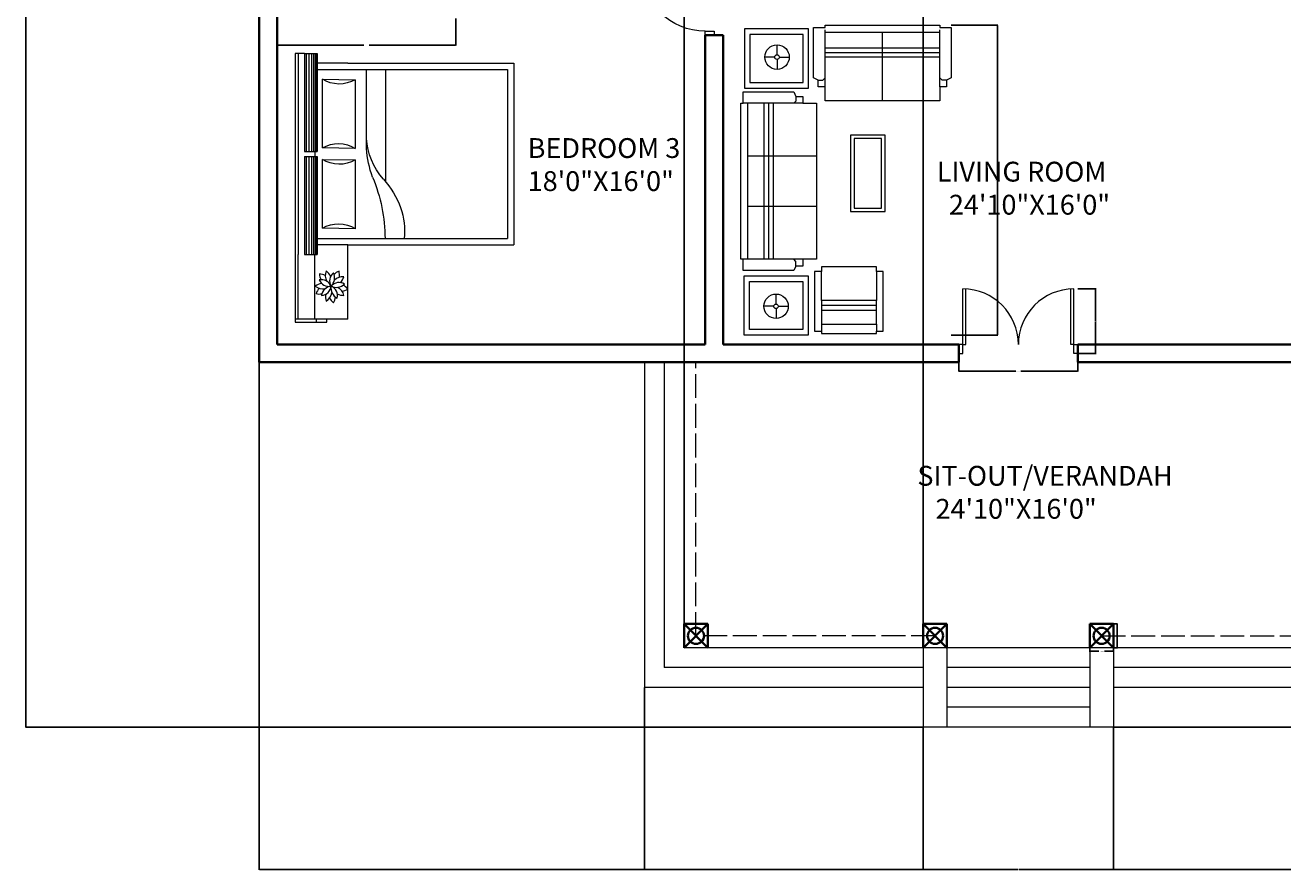
# Model space of a CAD drawing. Units: inches. Extents: x 4602 to 5612, y 5125 to 6591.
# Tile 1 of 6: x 4602 to 5237, y 5125 to 5551. Entities that reach past the tile are written whole.
import ezdxf

# ---------------------------------------------------------------- set-up
doc = ezdxf.new("R2010")
doc.units = ezdxf.units.IN
doc.linetypes.add('ACAD_ISO02W100', pattern=[15, 12, -3])
for name, color, linetype, lineweight in [('A-ANNO-DIMS', 2, 'Continuous', 18), ('A-AREA-IDEN', 7, 'Continuous', 18), ('A-COLS', 7, 'Continuous', 35), ('A-DOOR', 4, 'Continuous', 18), ('A-FLOR-EDGE', 7, 'Continuous', 18), ('A-FLOR-OVHD', 8, 'ACAD_ISO02W100', 13), ('A-FLOR-STRS', 7, 'Continuous', 18), ('A-FURN', 8, 'Continuous', 13), ('A-WALL', 7, 'Continuous', 35)]:
    doc.layers.add(name, color=color, linetype=linetype, lineweight=lineweight)
doc.styles.get("Standard").update_dxf_attribs({"font": 'arial.ttf'})
doc.dimstyles.get("Standard").update_dxf_attribs({"dimtxt": 0.18, "dimasz": 0.18, "dimexe": 0.18, "dimexo": 0.0625, "dimgap": 0.09, "dimtad": 0, "dimtih": 1, "dimtoh": 1, "dimdec": 4, "dimzin": 0, "dimdsep": 46, "dimtxsty": 'Standard', "dimcen": 0.09, "dimadec": 0, "dimazin": 0, "dimtfac": 1, "dimtdec": 4, "dimtofl": 0, "dimtmove": 0, "dimatfit": 3, "dimfxl": 1, "dimtolj": 1, "dimtzin": 0, "dimarcsym": 0})

# ---------------------------------------------------------------- blocks, each defined once
blk = doc.blocks.new('A$C1C981678')
for p, q in [((0, 1425), (0, 2066)), ((0, 2066), (591, 2066)), ((55, 1480), (55, 2011)), ((55, 2011), (536, 2011)), ((536, 2011), (536, 1480)), ((591, 2066), (591, 1425)), ((643, 1571), (643, 2074)), ((643, 2074), (757, 2074)), ((757, 2097), (2312, 2097)), ((757, 2074), (757, 2097)), ((757, 1571), (757, 2074)), ((757, 2028), (2312, 2028)), ((1283, 1342), (1283, 2028)), ((1786, 1342), (1786, 2028)), ((2312, 2097), (2312, 2074)), ((2312, 2074), (2426, 2074)), ((2312, 1571), (2312, 2074)), ((2426, 2074), (2426, 1571)), ((2463, 2062), (2463, 1422)), ((3055, 2062), (2463, 2062)), ((3055, 1422), (3055, 2062)), ((2519, 2007), (2519, 1477)), ((3000, 2007), (2519, 2007)), ((3000, 1477), (3000, 2007)), ((287, 1770), (287, 1869)), ((2312, 1868), (757, 1868)), ((2312, 1822), (757, 1822)), ((2312, 1777), (757, 1777)), ((2773, 1759), (2773, 1859)), ((264, 1747), (165, 1747)), ((287, 1724), (287, 1625)), ((310, 1747), (409, 1747)), ((2750, 1737), (2651, 1737)), ((2773, 1714), (2773, 1615)), ((2796, 1737), (2895, 1737)), ((689, 1548), (643, 1571)), ((689, 1479), (689, 1548)), ((689, 1548), (734, 1548)), ((734, 1548), (757, 1571)), ((757, 1479), (757, 1571)), ((2335, 1548), (2312, 1571)), ((2312, 1479), (2312, 1571)), ((2380, 1548), (2335, 1548)), ((2426, 1571), (2380, 1548)), ((2380, 1548), (2380, 1479)), ((591, 1425), (0, 1425)), ((536, 1480), (55, 1480)), ((757, 1479), (689, 1479)), ((757, 1342), (757, 1479)), ((2380, 1479), (2312, 1479)), ((2312, 1479), (2312, 1342)), ((2463, 1422), (3055, 1422)), ((2519, 1477), (3000, 1477)), ((17, 1295), (17, 746)), ((40, 1295), (17, 1295)), ((634, 1364), (40, 1364)), ((40, 1364), (40, 1295)), ((108, 1295), (40, 1295)), ((345, 1295), (108, 1295)), ((108, 1295), (108, 746)), ((245, 746), (245, 1295)), ((295, 746), (295, 1295)), ((345, 746), (345, 1295)), ((345, 1295), (634, 1295)), ((634, 1295), (634, 1364)), ((680, 1295), (634, 1295)), ((680, 746), (680, 1295)), ((2312, 1342), (757, 1342)), ((2337, 114), (2337, 1257)), ((2337, 1257), (2475, 1257)), ((2475, 1326), (2543, 1326)), ((2475, 1257), (2475, 1326)), ((2475, 1257), (2566, 1257)), ((2543, 1326), (2566, 1372)), ((2543, 1326), (2543, 1280)), ((2543, 1280), (2566, 1257)), ((2566, 1372), (3069, 1372)), ((2566, 1257), (3046, 1257)), ((2772, 114), (2772, 1257)), ((2817, 114), (2817, 1257)), ((2863, 114), (2863, 1257)), ((3023, 1257), (3023, 114)), ((3069, 1372), (3069, 1257)), ((3069, 1257), (3092, 1257)), ((3092, 1257), (3092, 114)), ((1995, 1003), (1232, 1003)), ((1232, 1003), (1232, 659)), ((1960, 969), (1266, 969)), ((1266, 969), (1266, 694)), ((1960, 694), (1960, 969)), ((1995, 659), (1995, 1003)), ((17, 746), (40, 746)), ((40, 746), (40, 678)), ((108, 746), (40, 746)), ((40, 678), (634, 678)), ((108, 746), (345, 746)), ((634, 746), (345, 746)), ((634, 746), (680, 746)), ((634, 678), (634, 746)), ((1232, 659), (1995, 659)), ((1266, 694), (1960, 694)), ((2337, 686), (3023, 686)), ((2475, 114), (2337, 114)), ((2475, 46), (2475, 114)), ((2475, 114), (2566, 114)), ((2543, 46), (2475, 46)), ((2543, 91), (2566, 114)), ((2543, 46), (2543, 91)), ((2566, 0), (2543, 46)), ((2566, 114), (3046, 114)), ((3069, 0), (2566, 0)), ((3092, 114), (3069, 114)), ((3069, 114), (3069, 0))]:
    blk.add_line(p, q)
for radius in [122, 22.9]:
    blk.add_circle((2773, 1737), radius)
for major_axis in [(-86.2, 86.2), (16.2, 16.2)]:
    blk.add_ellipse((287, 1747), major_axis=major_axis, ratio=1)
blk = doc.blocks.new('DOOR-PAIR-60IN')
for p, q in [((2, 4.5), (2, 32.5)), ((3.5, 4.5), (3.5, 32.46)), ((56.5, 4.5), (56.5, 32.46)), ((58, 4.5), (58, 32.5)), ((2, 4.5), (0, 4.5)), ((2, 0), (2, 4.5)), ((2, 4.5), (3.5, 4.5)), ((58, 4.5), (56.5, 4.5)), ((58, 0), (58, 4.5)), ((58, 4.5), (60, 4.5)), ((0, 0), (2, 0)), ((60, 0), (58, 0))]:
    blk.add_line(p, q)
for centre, start, end in [((2, 4.5), 0, 90), ((58, 4.5), 90, 180)]:
    blk.add_arc(centre, 28, start, end)
blk = doc.blocks.new('DOOR-36IN-DEEP-JAMB')
for p, q in [((2, 4.5), (2, 36.5)), ((3.5, 4.5), (3.5, 36.46)), ((0, 4.5), (2, 4.5)), ((2, 4.5), (2, 0)), ((2, 4.5), (3.5, 4.5)), ((36, 4.5), (34, 4.5)), ((34, 4.5), (34, 0)), ((2, 0), (0, 0)), ((34, 0), (36, 0))]:
    blk.add_line(p, q)
blk.add_arc((2, 4.5), 32, 0, 90)
blk = doc.blocks.new('POST-POOMUKHAM')
for p, q in [((12, 12), (0, 12)), ((0, 12), (0, 0)), ((12, 0), (0, 12)), ((0, 0), (12, 12)), ((12, 0), (12, 12))]:
    blk.add_line(p, q)
blk.add_circle((6, 6), 4.06)
blk = doc.blocks.new('BED-DOUBLE')
for p, q in [((0, 108.76), (49.36, 108.76)), ((49.36, 108.76), (52.03, 108.76)), ((52.03, 110.36), (101.4, 110.36)), ((52.03, 108.76), (101.4, 108.76)), ((0, 105.55), (49.36, 105.55)), ((0, 105.55), (0, 99.15)), ((0, 104.75), (49.36, 104.75)), ((0, 103.35), (49.36, 103.35)), ((0, 102.06), (49.36, 102.06)), ((49.36, 105.55), (49.36, 99.15)), ((52.03, 105.55), (52.03, 99.15)), ((52.03, 105.55), (101.4, 105.55)), ((52.03, 104.75), (101.4, 104.75)), ((52.03, 103.35), (101.4, 103.35)), ((52.03, 102.06), (101.4, 102.06)), ((101.4, 105.55), (101.4, 99.15)), ((0, 101), (49.36, 101)), ((0, 100.18), (49.36, 100.18)), ((0, 99.59), (49.36, 99.59)), ((0, 99.15), (49.36, 99.15)), ((4.8, 83.67), (4.8, 99.15)), ((8.01, 99.15), (8.01, 3.2)), ((47.64, 96.58), (12.95, 96.58)), ((12.95, 96.58), (13.21, 79.95)), ((47.9, 79.95), (47.64, 96.58)), ((49.36, 100.32), (52.03, 100.32)), ((52.03, 101), (101.4, 101)), ((52.03, 100.18), (101.4, 100.18)), ((52.03, 99.59), (101.4, 99.59)), ((52.03, 99.15), (101.4, 99.15)), ((88.11, 96.58), (53.42, 96.58)), ((53.42, 96.58), (53.67, 79.95)), ((88.36, 79.95), (88.11, 96.58)), ((93.39, 99.15), (93.39, 3.2)), ((96.59, 83.67), (96.59, 99.15)), ((4.8, 83.67), (4.8, 0)), ((96.59, 83.67), (96.59, 0)), ((13.21, 79.95), (47.9, 79.95)), ((53.67, 79.95), (88.36, 79.95)), ((48.03, 74.3), (8.01, 74.3)), ((64.45, 64.53), (8.01, 64.53)), ((4.8, 0), (96.59, 0)), ((8.01, 3.2), (93.39, 3.2))]:
    blk.add_line(p, q)
for centre, start, end in [((-0.76, 88.06), 329.87223, 31.87128), ((61.61, 88.48), 149.87223, 211.87128), ((39.71, 88.06), 329.87223, 31.87128), ((102.07, 88.48), 149.87223, 211.87128)]:
    blk.add_arc(centre, 16.15, start, end)
for centre, major_axis, ratio, start_param, end_param in [((41.23, 29.43), (0, -44.91), 0.84, 2.512571, 3.097265), ((44.48, 1.25), (0, -73.18), 0.84, 2.845884, 3.083884), ((93.61, 177.65), (0, -112.7), 0.84, -0.336035, -0.002349), ((86.52, 99.05), (13.81, -42.31), 0.868451, -0.988378, -0.183496)]:
    blk.add_ellipse(centre, major_axis=major_axis, ratio=ratio, start_param=start_param, end_param=end_param)
blk = doc.blocks.new('*D21')
at = {"layer": 'A-ANNO-DIMS', "color": 0, "lineweight": -2, "transparency": 16777216}
for p, q in [((5139.24, 5236.49), (5139.24, 5234.57)), ((5151.24, 5236.49), (5151.24, 5234.57)), ((5139.42, 5234.75), (5143.85, 5234.75)), ((5151.06, 5234.75), (5146.63, 5234.75))]:
    blk.add_line(p, q, dxfattribs=at)
at = {"layer": 'A-ANNO-DIMS', "color": 0, "transparency": 16777216}
for points in [[(5139.42, 5234.78), (5139.42, 5234.72), (5139.24, 5234.75)], [(5151.06, 5234.78), (5151.06, 5234.72), (5151.24, 5234.75)]]:
    blk.add_solid(points, dxfattribs=at)
at = {"layer": 'Defpoints', "color": 0, "transparency": 16777216}
for p in [(5139.24, 5236.55), (5151.24, 5236.55), (5151.24, 5234.75)]:
    blk.add_point(p, dxfattribs=at)
at = {"layer": 'A-ANNO-DIMS', "color": 0, "transparency": 16777216, "insert": (5145.24, 5234.75), "char_height": 0.18, "attachment_point": 5}
blk.add_mtext('\\A1;PORCH POST 12 TYP.', dxfattribs=at)
blk = doc.blocks.new('*D22')
at = {"layer": 'A-ANNO-DIMS', "color": 0, "lineweight": -2, "transparency": 16777216}
for p, q in [((5151.3, 5248.55), (5153.22, 5248.55)), ((5153.04, 5248.37), (5153.04, 5242.73)), ((5153.04, 5236.73), (5153.04, 5242.37)), ((5151.3, 5236.55), (5153.22, 5236.55))]:
    blk.add_line(p, q, dxfattribs=at)
at = {"layer": 'A-ANNO-DIMS', "color": 0, "transparency": 16777216}
for points in [[(5153.01, 5248.37), (5153.07, 5248.37), (5153.04, 5248.55)], [(5153.01, 5236.73), (5153.07, 5236.73), (5153.04, 5236.55)]]:
    blk.add_solid(points, dxfattribs=at)
at = {"layer": 'Defpoints', "color": 0, "transparency": 16777216}
for p in [(5151.24, 5248.55), (5153.04, 5248.55), (5151.24, 5236.55)]:
    blk.add_point(p, dxfattribs=at)
at = {"layer": 'A-ANNO-DIMS', "color": 0, "transparency": 16777216, "insert": (5153.04, 5242.55), "char_height": 0.18, "attachment_point": 5}
blk.add_mtext('\\A1;12 TYP.', dxfattribs=at)
blk = doc.blocks.new('*D29')
at = {"layer": 'A-ANNO-DIMS', "color": 0, "lineweight": -2, "transparency": 16777216}
for p, q in [((5073.24, 5384.99), (5073.24, 5375.87)), ((5133.24, 5384.99), (5133.24, 5375.87)), ((5073.42, 5376.05), (5101.97, 5376.05)), ((5133.06, 5376.05), (5104.5, 5376.05))]:
    blk.add_line(p, q, dxfattribs=at)
at = {"layer": 'A-ANNO-DIMS', "color": 0, "transparency": 16777216}
for points in [[(5073.42, 5376.08), (5073.42, 5376.02), (5073.24, 5376.05)], [(5133.06, 5376.08), (5133.06, 5376.02), (5133.24, 5376.05)]]:
    blk.add_solid(points, dxfattribs=at)
at = {"layer": 'Defpoints', "color": 0, "transparency": 16777216}
for p in [(5073.24, 5385.05), (5133.24, 5385.05), (5133.24, 5376.05)]:
    blk.add_point(p, dxfattribs=at)
at = {"layer": 'A-ANNO-DIMS', "color": 0, "transparency": 16777216, "insert": (5103.24, 5376.05), "char_height": 0.18, "attachment_point": 5}
blk.add_mtext('\\A1;DOOR PAIR 60 TYP.', dxfattribs=at)
blk = doc.blocks.new('*D30')
at = {"layer": 'A-ANNO-DIMS', "color": 0, "lineweight": -2, "transparency": 16777216}
for p, q in [((5133.3, 5417.55), (5142.42, 5417.55)), ((5142.24, 5417.37), (5142.24, 5401.48)), ((5142.24, 5385.23), (5142.24, 5401.12)), ((5133.3, 5385.05), (5142.42, 5385.05))]:
    blk.add_line(p, q, dxfattribs=at)
at = {"layer": 'A-ANNO-DIMS', "color": 0, "transparency": 16777216}
for points in [[(5142.21, 5417.37), (5142.27, 5417.37), (5142.24, 5417.55)], [(5142.21, 5385.23), (5142.27, 5385.23), (5142.24, 5385.05)]]:
    blk.add_solid(points, dxfattribs=at)
at = {"layer": 'Defpoints', "color": 0, "transparency": 16777216}
for p in [(5133.24, 5417.55), (5142.24, 5417.55), (5133.24, 5385.05)]:
    blk.add_point(p, dxfattribs=at)
at = {"layer": 'A-ANNO-DIMS', "color": 0, "transparency": 16777216, "insert": (5142.24, 5401.3), "char_height": 0.18, "attachment_point": 5}
blk.add_mtext('\\A1;33 TYP.', dxfattribs=at)
blk = doc.blocks.new('*D39')
at = {"layer": 'A-ANNO-DIMS', "color": 0, "lineweight": -2, "transparency": 16777216}
for p, q in [((4729.24, 5554.03), (4729.24, 5540.38)), ((4819.46, 5554.03), (4819.46, 5540.38)), ((4729.42, 5540.56), (4773.04, 5540.56)), ((4819.28, 5540.56), (4775.66, 5540.56))]:
    blk.add_line(p, q, dxfattribs=at)
at = {"layer": 'A-ANNO-DIMS', "color": 0, "transparency": 16777216}
for points in [[(4729.42, 5540.59), (4729.42, 5540.53), (4729.24, 5540.56)], [(4819.28, 5540.59), (4819.28, 5540.53), (4819.46, 5540.56)]]:
    blk.add_solid(points, dxfattribs=at)
at = {"layer": 'Defpoints', "color": 0, "transparency": 16777216}
for p in [(4729.24, 5554.09), (4819.46, 5554.09), (4819.46, 5540.56)]:
    blk.add_point(p, dxfattribs=at)
at = {"layer": 'A-ANNO-DIMS', "color": 0, "transparency": 16777216, "insert": (4774.35, 5540.56), "char_height": 0.18, "attachment_point": 5}
blk.add_mtext('\\A1;WARDROBE 90 TYP.', dxfattribs=at)
blk = doc.blocks.new('*D51')
at = {"layer": 'A-ANNO-DIMS', "color": 0, "lineweight": -2, "transparency": 16777216}
for p, q in [((5069.38, 5550.61), (5092.95, 5550.61)), ((5092.77, 5550.43), (5092.77, 5472.63)), ((5092.77, 5394.45), (5092.77, 5472.26)), ((5069.38, 5394.27), (5092.95, 5394.27))]:
    blk.add_line(p, q, dxfattribs=at)
at = {"layer": 'A-ANNO-DIMS', "color": 0, "transparency": 16777216}
for points in [[(5092.74, 5550.43), (5092.8, 5550.43), (5092.77, 5550.61)], [(5092.74, 5394.45), (5092.8, 5394.45), (5092.77, 5394.27)]]:
    blk.add_solid(points, dxfattribs=at)
at = {"layer": 'Defpoints', "color": 0, "transparency": 16777216}
for p in [(5069.32, 5550.61), (5092.77, 5550.61), (5069.32, 5394.27)]:
    blk.add_point(p, dxfattribs=at)
at = {"layer": 'A-ANNO-DIMS', "color": 0, "transparency": 16777216, "insert": (5092.77, 5472.44), "char_height": 0.18, "attachment_point": 5}
blk.add_mtext('\\A1;LIVING SEATING 156', dxfattribs=at)
blk = doc.blocks.new('*D56')
at = {"layer": 'A-ANNO-DIMS', "color": 0, "lineweight": -2, "transparency": 16777216}
for p, q in [((5061.18, 6438.55), (4602.21, 6438.55)), ((4602.39, 6438.37), (4602.39, 5817.73)), ((4602.39, 5196.73), (4602.39, 5817.37)), ((5055.18, 5196.55), (4602.21, 5196.55))]:
    blk.add_line(p, q, dxfattribs=at)
at = {"layer": 'A-ANNO-DIMS', "color": 0, "transparency": 16777216}
for points in [[(4602.36, 6438.37), (4602.42, 6438.37), (4602.39, 6438.55)], [(4602.36, 5196.73), (4602.42, 5196.73), (4602.39, 5196.55)]]:
    blk.add_solid(points, dxfattribs=at)
at = {"layer": 'Defpoints', "color": 0, "transparency": 16777216}
for p in [(4602.39, 6438.55), (5061.24, 6438.55), (5055.24, 5196.55)]:
    blk.add_point(p, dxfattribs=at)
at = {"layer": 'A-ANNO-DIMS', "color": 0, "transparency": 16777216, "insert": (4602.39, 5817.55), "char_height": 0.18, "attachment_point": 5}
blk.add_mtext('\\A1;1242', dxfattribs=at)
blk = doc.blocks.new('*D57')
at = {"layer": 'A-ANNO-DIMS', "color": 0, "lineweight": -2, "transparency": 16777216}
for p, q in [((4720.24, 5380.49), (4720.24, 5124.52)), ((5486.24, 5380.49), (5486.24, 5124.52)), ((4720.42, 5124.7), (5102.95, 5124.7)), ((5486.06, 5124.7), (5103.53, 5124.7))]:
    blk.add_line(p, q, dxfattribs=at)
at = {"layer": 'A-ANNO-DIMS', "color": 0, "transparency": 16777216}
for points in [[(4720.42, 5124.73), (4720.42, 5124.67), (4720.24, 5124.7)], [(5486.06, 5124.73), (5486.06, 5124.67), (5486.24, 5124.7)]]:
    blk.add_solid(points, dxfattribs=at)
at = {"layer": 'Defpoints', "color": 0, "transparency": 16777216}
for p in [(4720.24, 5380.55), (5486.24, 5380.55), (5486.24, 5124.7)]:
    blk.add_point(p, dxfattribs=at)
at = {"layer": 'A-ANNO-DIMS', "color": 0, "transparency": 16777216, "insert": (5103.24, 5124.7), "char_height": 0.18, "attachment_point": 5}
blk.add_mtext('\\A1;766', dxfattribs=at)
blk = doc.blocks.new('*D60')
at = {"layer": 'A-ANNO-DIMS', "color": 0, "lineweight": -2, "transparency": 16777216}
for p, q in [((4934.59, 5248.61), (4934.59, 6572.85)), ((4934.77, 6572.67), (4994.46, 6572.67)), ((5055.06, 6572.67), (4995.37, 6572.67)), ((5055.24, 5248.61), (5055.24, 6572.85))]:
    blk.add_line(p, q, dxfattribs=at)
at = {"layer": 'A-ANNO-DIMS', "color": 0, "transparency": 16777216}
for points in [[(4934.77, 6572.7), (4934.77, 6572.64), (4934.59, 6572.67)], [(5055.06, 6572.7), (5055.06, 6572.64), (5055.24, 6572.67)]]:
    blk.add_solid(points, dxfattribs=at)
at = {"layer": 'Defpoints', "color": 0, "transparency": 16777216}
for p in [(5055.24, 6572.67), (4934.59, 5248.55), (5055.24, 5248.55)]:
    blk.add_point(p, dxfattribs=at)
at = {"layer": 'A-ANNO-DIMS', "color": 0, "transparency": 16777216, "insert": (4994.91, 6572.67), "char_height": 0.18, "attachment_point": 5}
blk.add_mtext('\\A1;120.65', dxfattribs=at)
blk = doc.blocks.new('*D61')
at = {"layer": 'A-ANNO-DIMS', "color": 0, "lineweight": -2, "transparency": 16777216}
for p, q in [((5055.24, 5196.49), (5055.24, 5124.52)), ((5151.24, 5196.49), (5151.24, 5124.52)), ((5055.42, 5124.7), (5103.02, 5124.7)), ((5151.06, 5124.7), (5103.46, 5124.7))]:
    blk.add_line(p, q, dxfattribs=at)
at = {"layer": 'A-ANNO-DIMS', "color": 0, "transparency": 16777216}
for points in [[(5055.42, 5124.73), (5055.42, 5124.67), (5055.24, 5124.7)], [(5151.06, 5124.73), (5151.06, 5124.67), (5151.24, 5124.7)]]:
    blk.add_solid(points, dxfattribs=at)
at = {"layer": 'Defpoints', "color": 0, "transparency": 16777216}
for p in [(5055.24, 5196.55), (5151.24, 5196.55), (5151.24, 5124.7)]:
    blk.add_point(p, dxfattribs=at)
at = {"layer": 'A-ANNO-DIMS', "color": 0, "transparency": 16777216, "insert": (5103.24, 5124.7), "char_height": 0.18, "attachment_point": 5}
blk.add_mtext('\\A1;96', dxfattribs=at)
blk = doc.blocks.new('*D65')
at = {"layer": 'A-ANNO-DIMS', "color": 0, "lineweight": -2, "transparency": 16777216}
for p, q in [((4914.59, 5216.49), (4914.59, 5124.52)), ((5291.89, 5216.49), (5291.89, 5124.52)), ((4914.77, 5124.7), (5102.85, 5124.7)), ((5291.71, 5124.7), (5103.63, 5124.7))]:
    blk.add_line(p, q, dxfattribs=at)
at = {"layer": 'A-ANNO-DIMS', "color": 0, "transparency": 16777216}
for points in [[(4914.77, 5124.73), (4914.77, 5124.67), (4914.59, 5124.7)], [(5291.71, 5124.73), (5291.71, 5124.67), (5291.89, 5124.7)]]:
    blk.add_solid(points, dxfattribs=at)
at = {"layer": 'Defpoints', "color": 0, "transparency": 16777216}
for p in [(4914.59, 5216.55), (5291.89, 5216.55), (5291.89, 5124.7)]:
    blk.add_point(p, dxfattribs=at)
at = {"layer": 'A-ANNO-DIMS', "color": 0, "transparency": 16777216, "insert": (5103.24, 5124.7), "char_height": 0.18, "attachment_point": 5}
blk.add_mtext('\\A1;377.3', dxfattribs=at)
blk = doc.blocks.new('*D68')
at = {"layer": 'A-ANNO-DIMS', "color": 0, "lineweight": -2, "transparency": 16777216}
for p, q in [((5291.95, 5216.55), (5612.27, 5216.55)), ((5612.09, 5216.37), (5612.09, 5206.73)), ((5612.09, 5196.73), (5612.09, 5206.37)), ((5151.3, 5196.55), (5612.27, 5196.55))]:
    blk.add_line(p, q, dxfattribs=at)
at = {"layer": 'A-ANNO-DIMS', "color": 0, "transparency": 16777216}
for points in [[(5612.06, 5216.37), (5612.12, 5216.37), (5612.09, 5216.55)], [(5612.06, 5196.73), (5612.12, 5196.73), (5612.09, 5196.55)]]:
    blk.add_solid(points, dxfattribs=at)
at = {"layer": 'Defpoints', "color": 0, "transparency": 16777216}
for p in [(5291.89, 5216.55), (5612.09, 5216.55), (5151.24, 5196.55)]:
    blk.add_point(p, dxfattribs=at)
at = {"layer": 'A-ANNO-DIMS', "color": 0, "transparency": 16777216, "insert": (5612.09, 5206.55), "char_height": 0.18, "attachment_point": 5}
blk.add_mtext('\\A1;20', dxfattribs=at)

msp = doc.modelspace()

# ---------------------------------------------------------------- linework, layer by layer
at = {"layer": 'A-FLOR-EDGE'}
for p in [(4934.5878, 5380.5515), (5271.8903, 5236.5515)]:
    msp.add_line(p, (4934.5878, 5236.5515), dxfattribs=at)
at = {"layer": 'A-FLOR-OVHD'}
for p, q in [((4940.5878, 5242.5515), (4940.5878, 5380.5515)), ((5061.239, 5242.5515), (4940.5878, 5242.5515)), ((5145.239, 5242.5515), (5265.8903, 5242.5515))]:
    msp.add_line(p, q, dxfattribs=at)
at = {"layer": 'A-FLOR-STRS'}
for p, q in [((4914.5878, 5380.5515), (4914.5878, 5216.5515)), ((4924.5878, 5380.5515), (4924.5878, 5226.5515)), ((5055.239, 5236.5515), (5055.239, 5196.5515)), ((5067.239, 5236.5515), (5067.239, 5196.5515)), ((5139.239, 5236.5515), (5139.239, 5196.5515)), ((5151.239, 5236.5515), (5151.239, 5196.5515)), ((5055.239, 5226.5515), (4924.5878, 5226.5515)), ((5139.239, 5226.5515), (5067.239, 5226.5515)), ((5281.8903, 5226.5515), (5151.239, 5226.5515)), ((5055.239, 5216.5515), (4914.5878, 5216.5515)), ((5139.239, 5216.5515), (5067.239, 5216.5515)), ((5291.8903, 5216.5515), (5151.239, 5216.5515)), ((5139.239, 5206.5515), (5067.239, 5206.5515)), ((5151.239, 5196.5515), (5055.239, 5196.5515))]:
    msp.add_line(p, q, dxfattribs=at)
at = {"layer": 'A-FURN'}
for p, q in [((4738.299, 5536.3158), (4738.299, 5484.2835)), ((4743.1019, 5536.3158), (4738.299, 5536.3158)), ((4764.9822, 5402.3658), (4764.9822, 5439.7224)), ((4738.299, 5434.9194), (4738.299, 5400.7648)), ((4739.8999, 5402.3658), (4739.8999, 5434.9194)), ((4748.3319, 5402.3658), (4748.3319, 5434.9194)), ((4754.3089, 5402.3658), (4738.299, 5402.3658)), ((4738.299, 5400.7648), (4754.3089, 5400.7648)), ((4748.9723, 5402.3658), (4748.9723, 5400.7648)), ((4764.9822, 5402.3658), (4754.3089, 5402.3658)), ((4754.3089, 5400.7648), (4754.3089, 5402.3658))]:
    msp.add_line(p, q, dxfattribs=at)
for centre, radius, start, end in [((4759.699, 5424.243), 6.1502, 157.3987049, 206.867596), ((4750.1825, 5421.1509), 6.6708, 24.50685, 54.869898), ((4760.9779, 5421.6824), 5.2277, 129.7527301, 210.955319), ((4752.5928, 5423.1075), 5.6702, 313.4841271, 27.2239221), ((4761.9699, 5421.5314), 5.167, 106.7524299, 140.4913709), ((4752.4261, 5424.5023), 8.2936, 352.6485911, 13.7894849), ((4752.4923, 5413.6568), 6.6708, 96.50685, 126.8698981), ((4751.3763, 5416.5538), 5.6702, 25.4841271, 99.2239219), ((4755.3228, 5424.088), 5.2277, 201.7527301, 282.955319), ((4755.7729, 5424.9849), 5.167, 178.7524302, 212.4913711), ((4749.9982, 5416.8262), 8.2936, 64.6485913, 85.7894851), ((4760.4375, 5415.5607), 5.2277, 57.7527301, 138.9553191), ((4759.2017, 5423.9758), 5.6702, 241.4841269, 315.2239218), ((4762.4776, 5417.5683), 6.1502, 85.3987049, 134.8675963), ((4756.596, 5425.6635), 6.6708, 312.50685, 342.8698982), ((4760.6005, 5414.5705), 5.167, 34.75243, 68.491371), ((4752.4923, 5423.663), 6.1502, 229.3987049, 278.8675962), ((4756.5484, 5412.1452), 8.2936, 136.648591, 157.7894849), ((4750.5735, 5420.1584), 5.167, 250.7524301, 284.4913711), ((4757.2333, 5413.3716), 5.6702, 97.4841271, 171.2239219), ((4751.2874, 5419.4531), 5.2277, 273.7527299, 354.9553189), ((4760.3334, 5413.5377), 6.6708, 168.5068502, 198.8698979), ((4750.8169, 5416.6298), 6.1502, 301.3987049, 350.867596), ((4763.0244, 5416.9282), 8.2936, 208.6485909, 229.789485), ((4762.0697, 5417.9586), 5.6702, 169.484127, 243.2239218), ((4754.4484, 5414.1829), 5.2277, 345.75273, 66.955319), ((4753.5571, 5413.722), 5.167, 322.75243, 356.4913708), ((4762.8697, 5420.9583), 6.6708, 240.5068499, 270.8698979), ((4756.9881, 5412.8631), 6.1502, 13.3987048, 62.867596), ((4760.4767, 5424.5653), 8.2936, 280.6485909, 301.7894849)]:
    msp.add_arc(centre, radius, start, end, dxfattribs=at)
at = {"layer": 'A-WALL'}
for p, q in [((4720.239, 6208.5515), (4720.239, 5380.5515)), ((4729.239, 5581.5515), (4729.239, 5389.5515)), ((4945.239, 5545.5515), (4945.239, 5389.5515)), ((4954.239, 5545.5515), (4945.239, 5545.5515)), ((4954.239, 5545.5515), (4954.239, 5389.5515)), ((4945.239, 5389.5515), (4729.239, 5389.5515)), ((5073.239, 5389.5515), (4954.239, 5389.5515)), ((5073.239, 5380.5515), (5073.239, 5389.5515)), ((5252.239, 5389.5515), (5133.239, 5389.5515)), ((5133.239, 5380.5515), (5133.239, 5389.5515)), ((5073.239, 5380.5515), (4720.239, 5380.5515)), ((5486.239, 5380.5515), (5133.239, 5380.5515))]:
    msp.add_line(p, q, dxfattribs=at)

# ---------------------------------------------------------------- block references
at = {"layer": 'A-COLS'}
for p in [(4934.5877, 5236.552), (5055.239, 5236.552), (5139.239, 5236.552)]:
    msp.add_blockref('POST-POOMUKHAM', p, dxfattribs=at)
at = {"layer": 'A-DOOR', "extrusion": (0, 0, -1), "zscale": -1, "rotation": 270.0000000000028}
msp.add_blockref('DOOR-36IN-DEEP-JAMB', (-4949.7386, 5581.5516), dxfattribs=at)
at = {"layer": 'A-DOOR'}
msp.add_blockref('DOOR-PAIR-60IN', (5073.239, 5385.052), dxfattribs=at)
at = {"layer": 'A-FURN', "xscale": 0.0505668113949487, "yscale": 0.0505668113949487, "zscale": 0.0505668113949487, "rotation": 90}
msp.add_blockref('A$C1C981678', (5069.3208, 5394.2739), dxfattribs=at)
at = {"layer": 'A-FURN', "extrusion": (0, 0, -1), "zscale": -1, "rotation": 270.0000000000056}
msp.add_blockref('BED-DOUBLE', (-4848.6552, 5536.3159), dxfattribs=at)

# ---------------------------------------------------------------- texts
at = {"layer": 'A-AREA-IDEN', "char_height": 10, "attachment_point": 1}
for s, width, insert in [('BEDROOM 3\\P18\'0"X16\'0"', 88.287986, (4855.67, 5493.6152)), ('LIVING ROOM\\P  24\'10"X16\'0"', 127.373556, (5062.0948, 5481.7127)), ('SIT-OUT/VERANDAH            24\'10"X16\'0"', 155.345326, (5052.2853, 5328.3028))]:
    msp.add_mtext_dynamic_manual_height_columns(s, width=width, gutter_width=12.5, heights=[0], dxfattribs=dict(at, insert=insert))

# ---------------------------------------------------------------- dimensions: what is measured, and where the dimension line sits
at = {"layer": 'A-ANNO-DIMS'}
for base, p1, p2, override, picture, middle in [((5055.239, 6572.6716), (4934.5878, 5248.5515), (5055.239, 5248.5515), {"dimdec": 2, "dimlfac": 1, "dimrnd": 0, "dimzin": 0, "dimdsep": 46, "dimlunit": 2}, '*D60', (4994.9134, 6572.6716)), ((5486.239, 5124.7015), (4720.239, 5380.5515), (5486.239, 5380.5515), {"dimdec": 0, "dimlfac": 1, "dimrnd": 0, "dimzin": 0, "dimdsep": 46, "dimlunit": 2}, '*D57', (5103.239, 5124.7015)), ((5291.8903, 5124.7015), (4914.5878, 5216.5515), (5291.8903, 5216.5515), {"dimdec": 1, "dimlfac": 1, "dimrnd": 0, "dimzin": 0, "dimdsep": 46, "dimlunit": 2}, '*D65', (5103.239, 5124.7015)), ((5151.239, 5124.7015), (5055.239, 5196.5515), (5151.239, 5196.5515), {"dimdec": 0, "dimlfac": 1, "dimrnd": 0, "dimzin": 0, "dimdsep": 46, "dimlunit": 2}, '*D61', (5103.239, 5124.7015))]:
    dim = msp.add_linear_dim(base=base, p1=p1, p2=p2, dimstyle='Standard', override=override, dxfattribs=at)
    dim.commit()
    dim.dimension.update_dxf_attribs({"geometry": picture, "text_midpoint": middle})
for base, p1, p2, picture, middle in [((4602.389, 6438.5515), (5055.239, 5196.5515), (5061.239, 6438.5515), '*D56', (4602.389, 5817.5515)), ((5612.089, 5216.5515), (5151.239, 5196.5515), (5291.8903, 5216.5515), '*D68', (5612.089, 5206.5515))]:
    dim = msp.add_linear_dim(base=base, p1=p1, p2=p2, angle=90, dimstyle='Standard', override={"dimdec": 0, "dimlfac": 1, "dimrnd": 0, "dimzin": 0, "dimdsep": 46, "dimlunit": 2}, dxfattribs=at)
    dim.commit()
    dim.dimension.update_dxf_attribs({"geometry": picture, "text_midpoint": middle})
for base, p1, p2, text, picture, middle in [((4819.4613, 5540.5608), (4729.239, 5554.0942), (4819.4613, 5554.0942), 'WARDROBE <> TYP.', '*D39', (4774.3502, 5540.5608)), ((5133.239, 5376.0515), (5073.239, 5385.0515), (5133.239, 5385.0515), 'DOOR PAIR <> TYP.', '*D29', (5103.239, 5376.0515)), ((5151.239, 5234.7515), (5139.239, 5236.5515), (5151.239, 5236.5515), 'PORCH POST <> TYP.', '*D21', (5145.239, 5234.7515))]:
    dim = msp.add_linear_dim(base=base, p1=p1, p2=p2, text=text, dimstyle='Standard', override={"dimdec": 0, "dimlfac": 1, "dimrnd": 0, "dimzin": 0, "dimdsep": 46, "dimlunit": 2}, dxfattribs=at)
    dim.commit()
    dim.dimension.update_dxf_attribs({"geometry": picture, "text_midpoint": middle})
for base, p1, p2, text, picture, middle in [((5092.7719, 5550.6143), (5069.3208, 5394.2739), (5069.3208, 5550.6143), 'LIVING SEATING <>', '*D51', (5092.7719, 5472.4441)), ((5142.2390416823, 5417.5515203146), (5133.2390416823, 5385.0515203146), (5133.2390416823, 5417.5515203146), '<> TYP.', '*D30', (5142.2390416823, 5401.3015203146)), ((5153.039, 5248.5515), (5151.239, 5236.5515), (5151.239, 5248.5515), '<> TYP.', '*D22', (5153.039, 5242.5515))]:
    dim = msp.add_linear_dim(base=base, p1=p1, p2=p2, angle=90, text=text, dimstyle='Standard', override={"dimdec": 0, "dimlfac": 1, "dimrnd": 0, "dimzin": 0, "dimdsep": 46, "dimlunit": 2}, dxfattribs=at)
    dim.commit()
    dim.dimension.update_dxf_attribs({"geometry": picture, "text_midpoint": middle})

doc.saveas('drawing.dxf')
